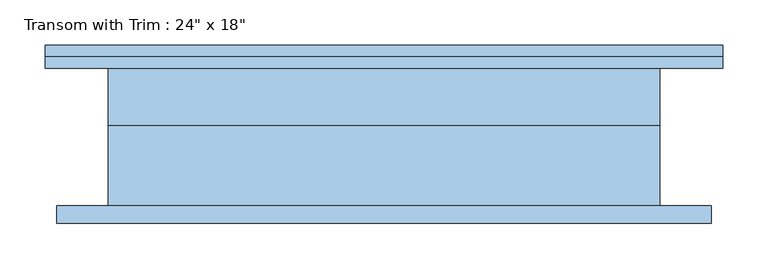
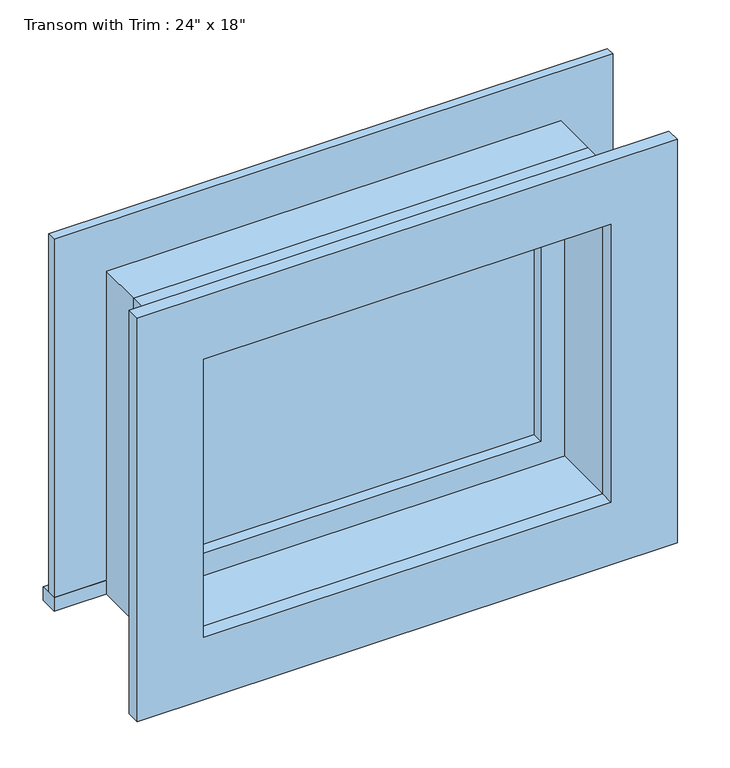
"""IFC4 building model written with IfcOpenShell, lengths in millimetres: window geometry."""

from ifc_helpers import new_model, si_unit, frame, origin, place, context, project, spatial, polyline, outline, extrude, source, transform, mapped, element, save


def window_8f6a5eb6(model_context):
    return source(origin(), model_context, "Body", "SweptSolid", [
        extrude(outline(polyline([(-412.75, 101.6), (336.55, 101.6), (336.55, 76.2), (-412.75, 76.2), (-412.75, 101.6)])), frame((0.0, 0.0, 2159.0), z_axis=(0.0, 0.0, 1.0), x_axis=(1.0, 0.0, 0.0)), (0.0, 0.0, 1.0), 19.05),
        extrude(outline(polyline([(2597.15, -323.85), (2597.15, 247.65), (2178.05, 247.65), (2178.05, 336.55), (2686.05, 336.55), (2686.05, -412.75), (2178.05, -412.75), (2178.05, -323.85), (2597.15, -323.85)])), frame((0.0, 76.2, 0.0), z_axis=(0.0, 1.0, 0.0), x_axis=(0.0, 0.0, 1.0)), (0.0, 0.0, 1.0), 12.7),
        extrude(outline(polyline([(2673.35, 323.85), (2673.35, -400.05), (2101.85, -400.05), (2101.85, 323.85), (2673.35, 323.85)]), holes=[polyline([(2584.45, 234.95), (2190.75, 234.95), (2190.75, -311.15), (2584.45, -311.15), (2584.45, 234.95)])]), frame((0.0, -95.25, 0.0), z_axis=(0.0, 1.0, 0.0), x_axis=(0.0, 0.0, 1.0)), (0.0, 0.0, 1.0), 19.05),
        extrude(outline(polyline([(203.2, 28.575), (-279.4, 28.575), (-279.4, 41.275), (203.2, 41.275), (203.2, 28.575)])), frame((0.0, 0.0, 2222.5), z_axis=(0.0, 0.0, 1.0), x_axis=(1.0, 0.0, 0.0)), (0.0, 0.0, 1.0), 330.2),
        extrude(outline(polyline([(2597.15, -323.85), (2178.05, -323.85), (2178.05, 247.65), (2597.15, 247.65), (2597.15, -323.85)]), holes=[polyline([(2552.7, -279.4), (2552.7, 203.2), (2222.5, 203.2), (2222.5, -279.4), (2552.7, -279.4)])]), frame((0.0, 12.7, 0.0), z_axis=(0.0, 1.0, 0.0), x_axis=(0.0, 0.0, 1.0)), (0.0, 0.0, 1.0), 44.45),
        extrude(outline(polyline([(2616.2, -342.9), (2159.0, -342.9), (2159.0, 266.7), (2616.2, 266.7), (2616.2, -342.9)]), holes=[polyline([(2584.45, -311.15), (2584.45, 234.95), (2190.75, 234.95), (2190.75, -311.15), (2584.45, -311.15)])]), frame((0.0, -76.2, 0.0), z_axis=(0.0, 1.0, 0.0), x_axis=(0.0, 0.0, 1.0)), (0.0, 0.0, 1.0), 88.9),
        extrude(outline(polyline([(2616.2, 266.7), (2616.2, -342.9), (2159.0, -342.9), (2159.0, 266.7), (2616.2, 266.7)]), holes=[polyline([(2597.15, 247.65), (2178.05, 247.65), (2178.05, -323.85), (2597.15, -323.85), (2597.15, 247.65)])]), frame((0.0, 12.7, 0.0), z_axis=(0.0, 1.0, 0.0), x_axis=(0.0, 0.0, 1.0)), (0.0, 0.0, 1.0), 63.5),
    ])


if __name__ == "__main__":
    model = new_model("IFC4")
    model_context = context("Model", 3, world=origin())
    ifc_project = project(units=[si_unit("LENGTHUNIT", "METRE", prefix="MILLI")], contexts=[model_context])
    site = spatial("IfcSite", under=ifc_project)
    building = spatial("IfcBuilding", under=site)
    placement = place(None, origin())
    window_shape = window_8f6a5eb6(model_context)
    element("IfcWindow", 1, ObjectType="Transom with Trim : 24\" x 18\"", at=placement, inside=building, context=model_context, shape_type="MappedRepresentation", body=[
        mapped(window_shape, transform((0.0, 0.0, 0.0), x_axis=(1.0, 0.0, 0.0), y_axis=(0.0, 1.0, 0.0), z_axis=(0.0, 0.0, 1.0))),
    ])
    save(model, "model.ifc")

# Revit data of these elements
# Type "Transom with Trim : 24\" x 18\""
#   Type Mark = "18"
#   Construction Type Id = "GSP4R"
#   Assembly Code = "B2020100"
#   Analytic Construction = "1/8 in Pilkington single glazing"
#   Visual Light Transmittance = 0.9
#   Solar Heat Gain Coefficient = 0.78
#   Heat Transfer Coefficient (U) = 0.6496 BTU/(h·ft²·°F)
#   Height = 1' - 6"
#   Default Sill Height = 7' - 1"
#   Trim Projection - Ext. = 0' - 0 1/2"
#   Trim Projection - Int. = 0' - 0 3/4"
#   Trim Width - Exterior = 0' - 3 1/2"
#   Trim Width - Interior = 0' - 3 1/2"
#   Width = 2' - 0"
#   Window Inset = 0' - 0 3/4"
#   Define Thermal Properties by = 1
#   Glass Pane Material = Glass
#   Sash Material = Sash
#   Trim Exterior Material = Trim
#   Trim Interior Material = Trim
#   Wall Closure = (empty or 0)
# Element 1 (IfcWindow, "Transom with Trim : 24\" x 18\"")
#   Materials on its faces: "Sash", "Trim", "Glass"
# Materials
#   "Glass": class "Glass", colour RGB 0 128 192, transparency 0.75, Description = "Soda Lime Glass", Cost = 0
#   "Sash": class "Wood", colour RGB 224 178 126, transparency 0
#   "Trim": class "Wood", colour RGB 224 178 126, transparency 0
